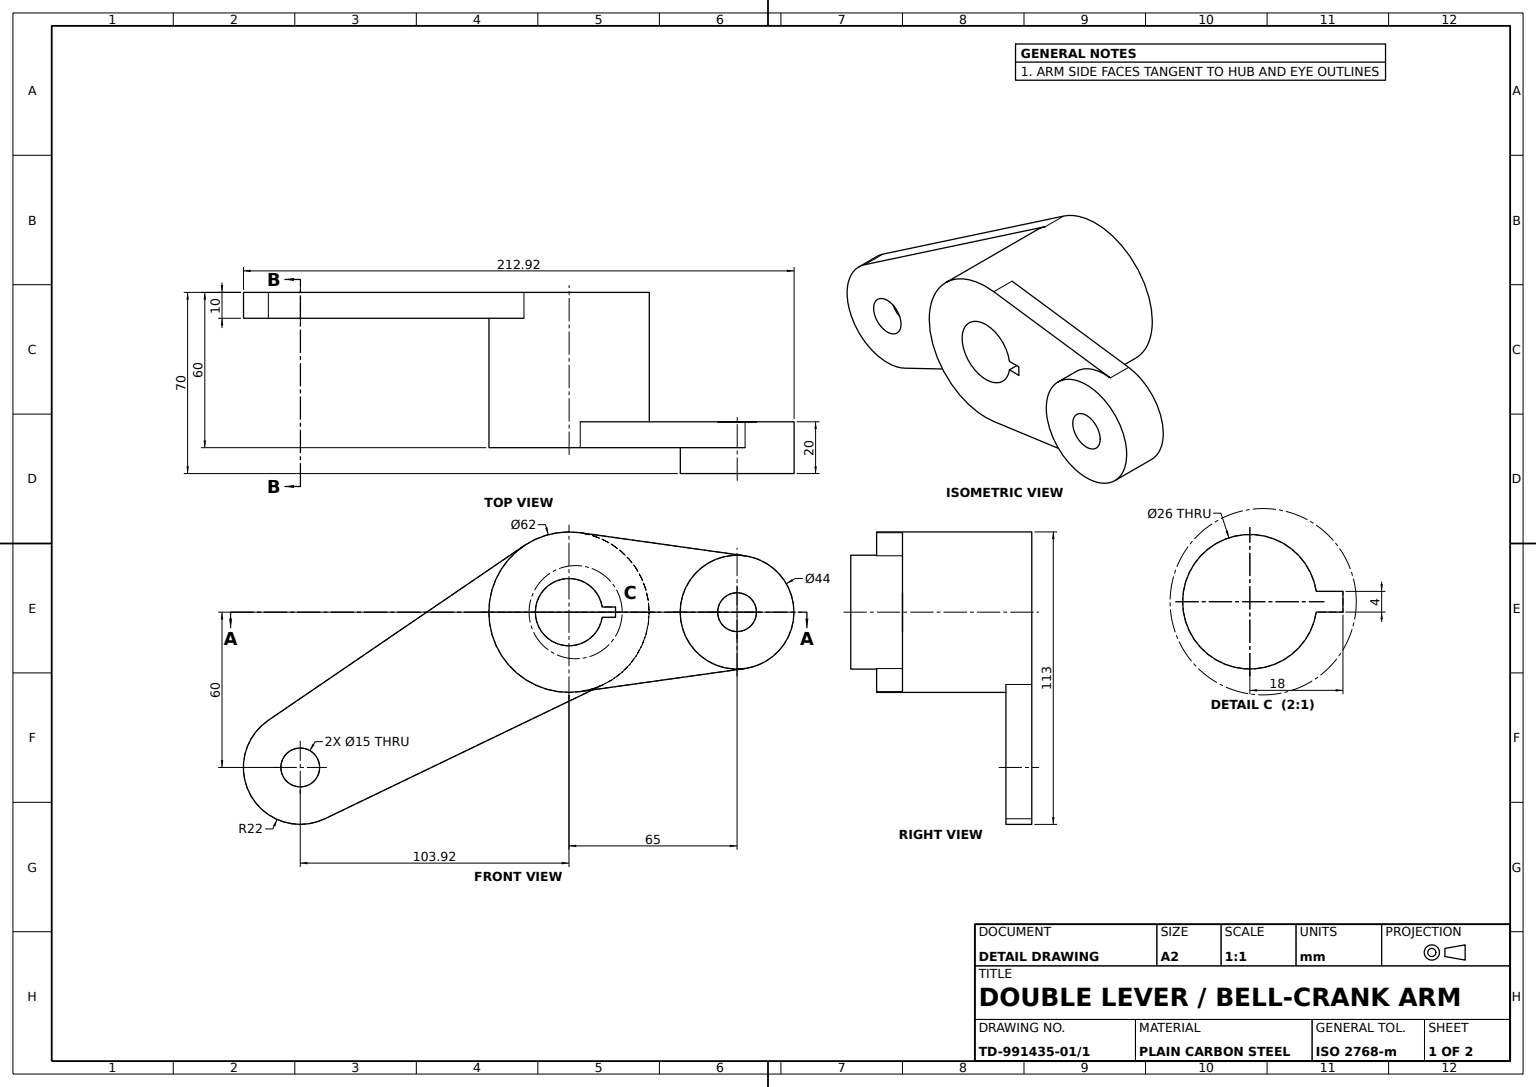
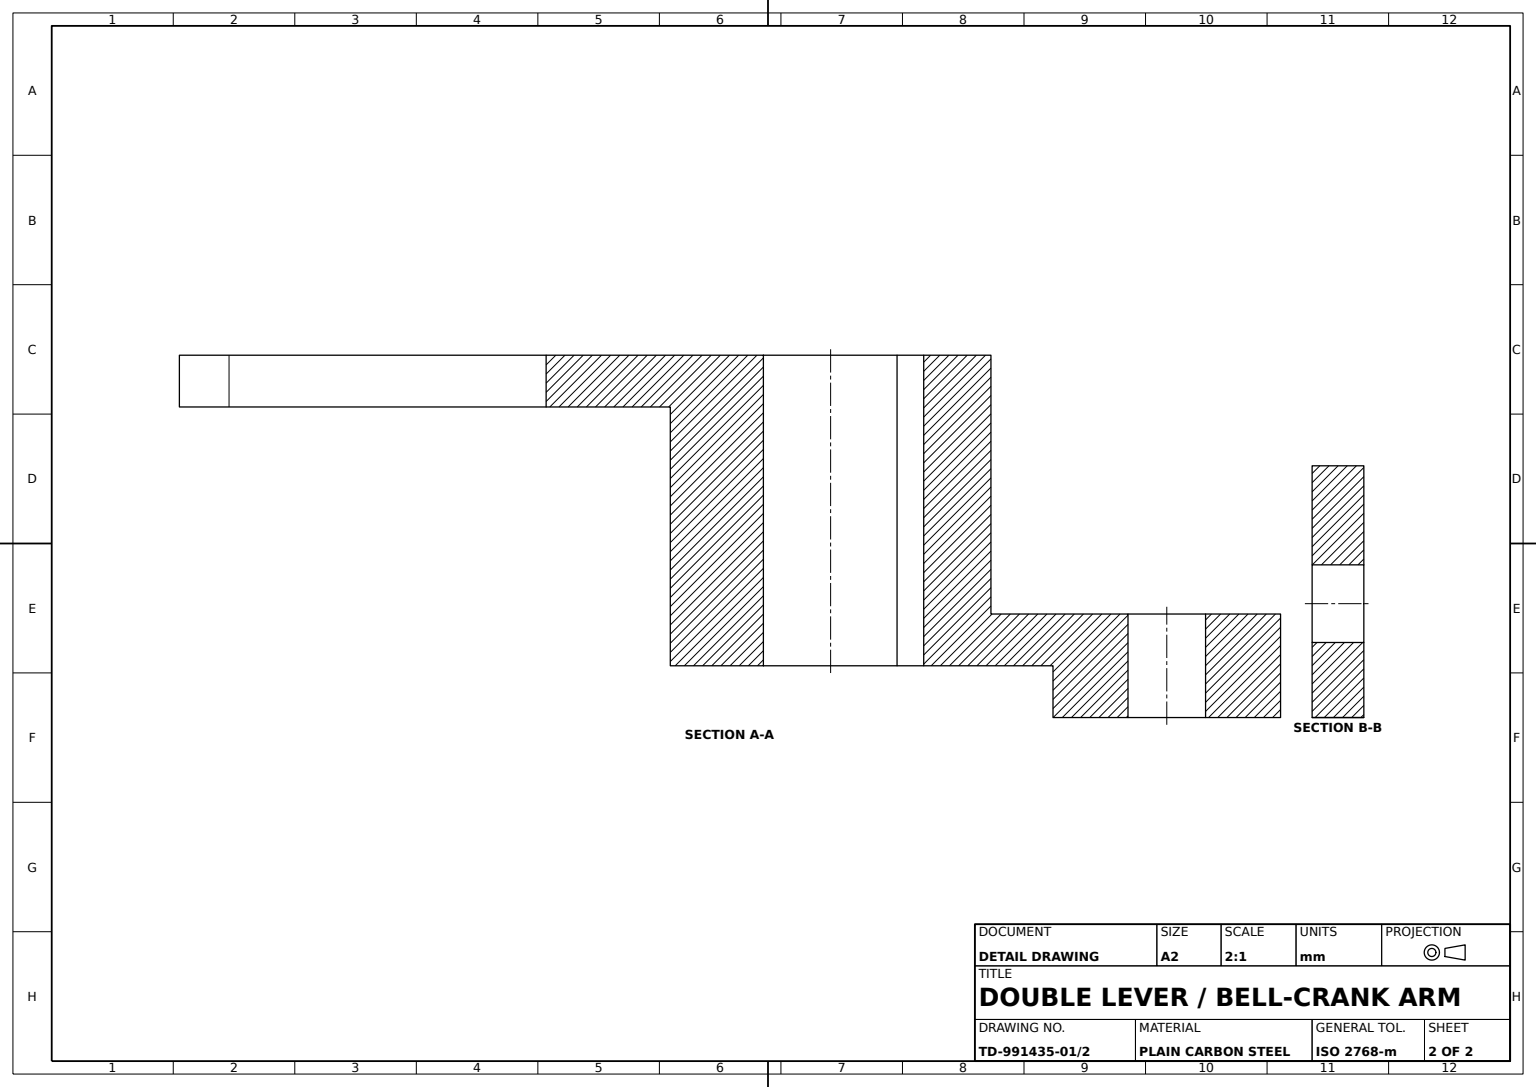
from build123d import *
from build123d.topology import SkipClean

# Parameters (mm, degrees)
ARM_PLATE_DEPTH        = 10
HUB_START              = -20
HUB_BOSS_PROFILE_R     = 22
HUB_BOSS_PROFILE_R_2   = 7.5
HUB_BOSS_DEPTH         = 20
ARM_HOLE_DEPTH         = 95.498677239
ARM_HOLE_DEPTH_BACK    = 95.498677239
ARM_HOLE_PROFILE_R     = 7.5
HUB_HOUSING_PROFILE_R  = 31
HUB_HOUSING_DEPTH      = 40
KEYED_BORE_DEPTH       = 101.647901121
KEYED_BORE_DEPTH_BACK  = 101.647901121
ANGLED_ARM_PROFILE_R   = 7.5
ANGLED_ARM_PLATE_DEPTH = 10


with BuildPart() as part:
    # Arm Plate Profile → Arm Plate (new body)
    with BuildSketch(Plane.XY):
        with BuildLine():
            Line((4.292307692, 30.701402161), (68.046153846, 21.788091856))
            ThreePointArc((68.046153846, 21.788091856), (87, 0), (68.046153846, -21.788091856))
            Line((68.046153846, -21.788091856), (4.292307692, -30.701402161))
            ThreePointArc((4.292307692, -30.701402161), (-31, 0), (4.292307692, 30.701402161))
        make_face()
    extrude(amount=-ARM_PLATE_DEPTH)

    # Hub Boss Profile → Hub Boss (add)
    with SkipClean():  # the faces are left unmerged after this step: merging them gives an invalid solid
        with BuildSketch(Plane(origin=(0, 0, -10), x_dir=(-1, 0, 0), z_dir=(0, 0, -1)).offset(HUB_START)):
            with Locations(Location((-65, 0, 0), (0, 0, 262.041168118))):
                Circle(HUB_BOSS_PROFILE_R)
            with Locations((-65, 0)):
                Circle(HUB_BOSS_PROFILE_R_2, mode=Mode.SUBTRACT)
        extrude(amount=HUB_BOSS_DEPTH)

    # Arm Hole Profile → Arm Hole (cut, two sides: drawn at the far end of the back side and taken through both)
    with SkipClean():  # the faces are left unmerged after this step: merging them gives an invalid solid
        with BuildSketch(Plane(origin=(0, 0, -10), x_dir=(-1, 0, 0), z_dir=(0, 0, -1)).offset(-ARM_HOLE_DEPTH_BACK)):
            with Locations((-65, 0)):
                Circle(ARM_HOLE_PROFILE_R)
        extrude(amount=ARM_HOLE_DEPTH + ARM_HOLE_DEPTH_BACK, mode=Mode.SUBTRACT)

    # Hub Housing Profile → Hub Housing (add)
    with SkipClean():  # the faces are left unmerged after this step: merging them gives an invalid solid
        with BuildSketch(Plane(origin=(0, 0, -10), x_dir=(-1, 0, 0), z_dir=(0, 0, -1))):
            with Locations(Location((0, 0, 0), (0, 0, 97.958831882))):
                Circle(HUB_HOUSING_PROFILE_R)
            with BuildLine():
                Line((-12.845232579, -2), (-18, -2))
                Line((-18, -2), (-18, 2))
                Line((-18, 2), (-12.845232579, 2))
                ThreePointArc((-12.845232579, 2), (13, 0), (-12.845232579, -2))
            make_face(mode=Mode.SUBTRACT)
        extrude(amount=HUB_HOUSING_DEPTH)

    # Keyed Bore Profile → Keyed Bore (cut, two sides: drawn at the far end of the back side and taken through both)
    with SkipClean():  # the faces are left unmerged after this step: merging them gives an invalid solid
        with BuildSketch(Plane(origin=(0, 0, -10), x_dir=(-1, 0, 0), z_dir=(0, 0, -1)).offset(-KEYED_BORE_DEPTH_BACK)):
            with BuildLine():
                Line((-18, -2), (-12.845232579, -2))
                ThreePointArc((-12.845232579, -2), (13, 0), (-12.845232579, 2))
                Line((-12.845232579, 2), (-18, 2))
                Line((-18, 2), (-18, -2))
            make_face()
        extrude(amount=KEYED_BORE_DEPTH + KEYED_BORE_DEPTH_BACK, mode=Mode.SUBTRACT)

    # Angled Arm Profile → Angled Arm Plate (add)
    with SkipClean():  # the faces are left unmerged after this step: merging them gives an invalid solid
        with BuildSketch(Plane.XY.offset(-50)):
            with BuildLine():
                Line((-17.469853837, 25.608674447), (-116.321009242, -41.826102006))
                ThreePointArc((-116.321009242, -41.826102006), (-122.975607337, -71), (-94.382971499, -79.823897994))
                Line((-94.382971499, -79.823897994), (13.442835709, -27.933674447))
                ThreePointArc((13.442835709, -27.933674447), (26.846787517, 15.5), (-17.469853837, 25.608674447))
            make_face()
            with Locations((-103.923048454, -60)):
                Circle(ANGLED_ARM_PROFILE_R, mode=Mode.SUBTRACT)
            with BuildLine():
                Line((18, -2), (18, 2))
                Line((18, 2), (12.845232579, 2))
                ThreePointArc((12.845232579, 2), (-13, 0), (12.845232579, -2))
                Line((12.845232579, -2), (18, -2))
            make_face(mode=Mode.SUBTRACT)
        extrude(amount=-ANGLED_ARM_PLATE_DEPTH)


solid = part.part
